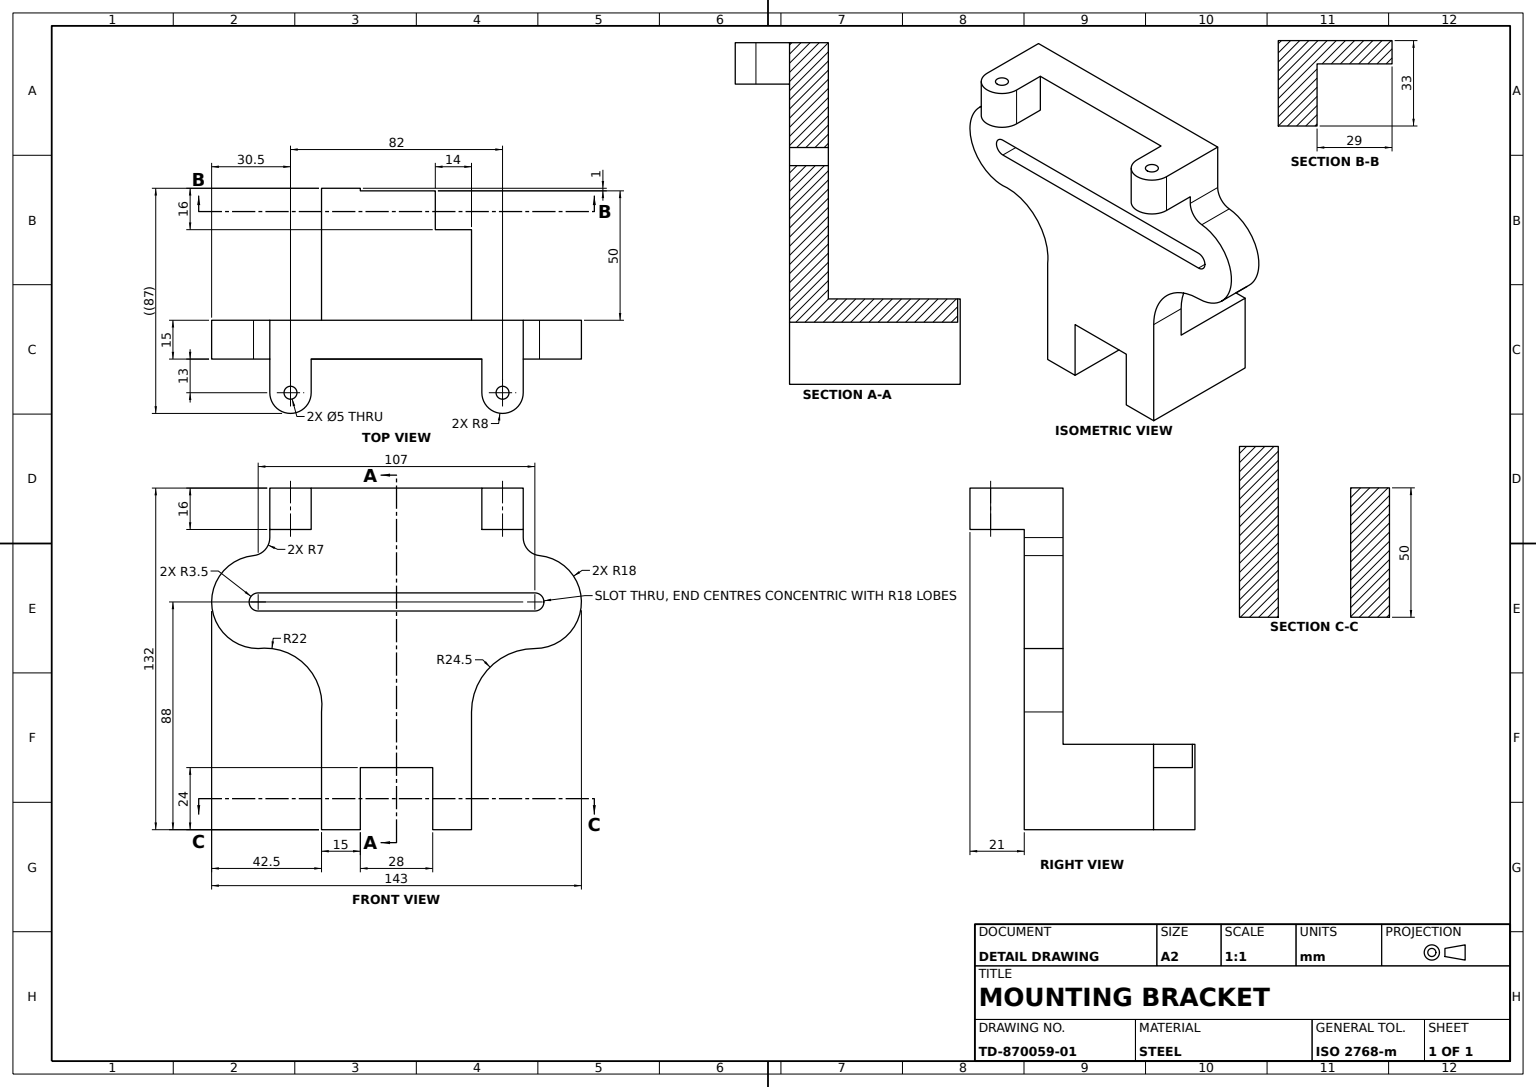
SolidWorks part; units mm, degrees
material "Plain Carbon Steel"
ref_plane "Front Plane" through (0, 0, 0) normal (0, 0, 1) x (1, 0, 0)
ref_plane "Top Plane" through (0, 0, 0) normal (0, 1, 0) x (1, 0, 0)
ref_plane "Right Plane" through (0, 0, 0) normal (1, 0, 0) x (0, 0, -1)
sketch "Base Plate Profile Sketch" plane through (0, 0, 0) normal (0, 0, 1) x (1, 0, 0)
  line L0 (0, 0) -> (98, 0)
  line L1 (98, 0) -> (98, -16)
  line L2 (0, 0) -> (0, -16)
  line L3 (49, 0) -> (49, -44)
  line L4 (34, -108) -> (64, -108)
  line L5 (49, -44) -> (102.5, -44)
  line L6 (49, -44) -> (-4.5, -44)
  line L7 (20, -132) -> (34, -132)
  line L8 (78, -132) -> (78, -86.5)
  line L9 (20, -132) -> (20, -86.5)
  line L10 (98, -16) -> (98, -19.1253)
  line L11 (0, -16) -> (0, -19.1253)
  line L12 (20, -132) -> (34, -132)
  line L13 (34, -132) -> (34, -108)
  line L14 (78, -86.5) -> (20, -86.5)
  line L15 (78, -132) -> (78, -108)
  line L17 (64, -108) -> (64, -132)
  line L18 (64, -132) -> (78, -132)
  arc A0 (-6.3, -26.0902) -> (-2.1679, -61.8483) centre (-4.5, -44) ccw
  arc A1 (102.5, -62) -> (104.3, -26.0902) centre (102.5, -44) ccw
  arc A2 (-4.5, -62) -> (-2.1679, -61.8483) centre (-1.9078, -83.8467) cw
  arc A3 (102.5, -62) -> (78, -86.5) centre (102.5, -86.5) ccw
  arc A4 (-6.3, -26.0902) -> (0, -19.1253) centre (-7, -19.1253) ccw
  arc A5 (104.3, -26.0902) -> (98, -19.1253) centre (105, -19.1253) cw
  arc A6 (-2.1679, -61.8483) -> (20, -86.5) centre (-1.8393, -83.8458) cw
  dimension "D8" = 18
  dimension "D9" = 7
  dimension "D11" = 22
  dimension "D12" = 14
  dimension "D14" = 24
  dimension "D4" = 18
  dimension "D17" = 24.5
  dimension "D19" = 22
  dimension "D1" = 98
  dimension "D2" = 16
  dimension "D3" = 16
  dimension "D5" = 108
  dimension "D6" = 53.5
  dimension "D7" = 53.5
  dimension "D10" = 88
  dimension "D13" = 24
  dimension "D15" = 14
  dimension "D16" = 46.1517
  dimension "D18" = 44
extrude "Base Plate" add sketch "Base Plate Profile Sketch" along normal blind 15
sketch "Long Slot Sketch" plane through (0, 0, 15) normal (0, 0, 1) x (1, 0, 0)
  line L0 (-4.5, -44) -> (102.5, -44)
  line L1 (-4.5, -40.5) -> (102.5, -40.5)
  line L2 (-4.5, -47.5) -> (102.5, -47.5)
  arc A0 (-4.5, -40.5) -> (-4.5, -47.5) centre (-4.5, -44) ccw
  arc A1 (102.5, -47.5) -> (102.5, -40.5) centre (102.5, -44) ccw
  dimension "D1" = 7
  dimension "D2" = 7
  dimension "D3" = 107
  dimension "D4" = 107
extrude "Long Slot" cut sketch "Long Slot Sketch" against normal blind 15
sketch "Lower Block Sketch" plane through (20, 0, 0) normal (-1, 0, 0) x (0, 0, 1)
  line L0 (15, -132) -> (15, -99)
  line L1 (15, -132) -> (15, -86.5) construction
  line L2 (15, -99) -> (-51, -99)
  line L3 (-51, -99) -> (-51, -132)
  line L4 (-51, -132) -> (15, -132)
  dimension "D1" = 33
  dimension "D2" = 66
extrude "Lower Block 33x66" add sketch "Lower Block Sketch" against normal blind 15
sketch "Block Extension Sketch" plane through (0, 0, 0) normal (0, 0, -1) x (-1, 0, 0)
  line L0 (-35, -99) -> (-64, -99)
  line L1 (-64, -99) -> (-64, -108)
  line L2 (-64, -108) -> (-35, -108)
  line L3 (-35, -108) -> (-35, -99)
extrude "Block Extension" add sketch "Block Extension Sketch" along normal blind 50
sketch "Block End Sketch" plane through (78, 0, 0) normal (1, 0, 0) x (0, 0, -1)
  line L0 (-15, -132) -> (-15, -99)
  line L1 (-15, -132) -> (-15, -86.5) construction
  line L2 (-15, -99) -> (35, -99)
  line L3 (50, -99) -> (0, -99) construction
  line L4 (35, -99) -> (35, -132)
  line L5 (51, -132) -> (-15, -132) construction
  line L6 (35, -132) -> (-15, -132)
  dimension "D1" = 50
  dimension "D2" = 50
extrude "Block End 50x50" add sketch "Block End Sketch" against normal blind 15
sketch "Lug A Sketch" plane through (0, 0, 0) normal (0, 1, 0) x (1, 0, 0)
  line L0 (0, -15) -> (16, -15)
  line L1 (0, -15) -> (98, -15) construction
  line L2 (8, -15) -> (8, -28)
  line L3 (0, -15) -> (0, -28)
  line L4 (16, -15) -> (16, -28)
  arc A0 (0, -28) -> (16, -28) centre (8, -28) ccw
  dimension "D3" = 8
  dimension "D1" = 16
  dimension "D2" = 13
  dimension "D4" = 13
  dimension "D5" = 13
extrude "Lug A" add sketch "Lug A Sketch" against normal blind 16
sketch "Lug B Sketch" plane through (0, 0, 0) normal (0, 1, 0) x (1, 0, 0)
  line L0 (98, -15) -> (82, -15)
  line L1 (16, -15) -> (98, -15) construction
  line L2 (90, -15) -> (90, -28)
  line L3 (82, -15) -> (82, -28)
  line L4 (98, -15) -> (98, -28)
  arc A0 (82, -28) -> (98, -28) centre (90, -28) ccw
  dimension "D3" = 8
  dimension "D1" = 16
  dimension "D2" = 13
  dimension "D4" = 13
  dimension "D5" = 13
extrude "Lug B" add sketch "Lug B Sketch" against normal blind 16
sketch "Lug Holes Sketch" plane through (0, -16, 0) normal (0, -1, 0) x (1, 0, 0)
  circle A0 centre (90, 28) radius 2.5
  circle A1 centre (8, 28) radius 2.5
  dimension "D1" = 5
  dimension "D2" = 5
extrude "Lug Holes 2x5mm" cut sketch "Lug Holes Sketch" against normal blind 16
